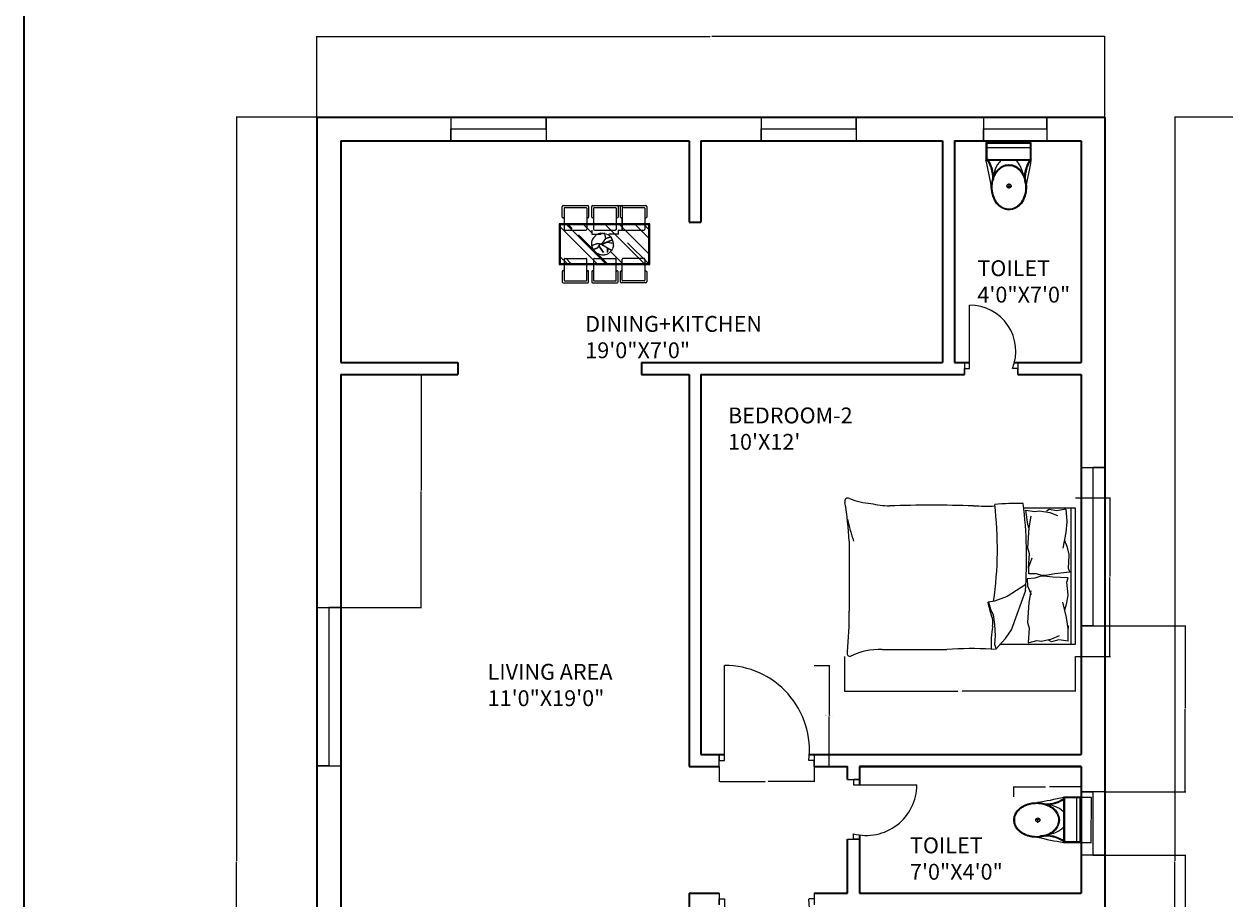
# Model space of a CAD drawing. Units: inches. Extents: x 2416 to 3391, y 1375 to 2496.
# Tile 2 of 13: x 2416 to 2871, y 1738 to 2069. Entities that reach past the tile are written whole.
import ezdxf

# ---------------------------------------------------------------- set-up
doc = ezdxf.new("R2010")
doc.units = ezdxf.units.IN
for name, color, linetype, lineweight in [('A-ANNO-DIMS', 2, 'Continuous', 18), ('A-ANNO-TTLB', 7, 'Continuous', 35), ('A-AREA-IDEN', 7, 'Continuous', 18), ('A-DOOR', 3, 'Continuous', 20), ('A-FLOR-FIXT', 9, 'Continuous', 18), ('A-FURN', 8, 'Continuous', 18), ('A-FURN-PATT', 252, 'Continuous', 13), ('A-GLAZ', 4, 'Continuous', 18), ('A-WALL', 7, 'Continuous', 35)]:
    doc.layers.add(name, color=color, linetype=linetype, lineweight=lineweight)
doc.styles.get("Standard").update_dxf_attribs({"font": 'arial.ttf'})
doc.dimstyles.get("Standard").update_dxf_attribs({"dimtxt": 0.18, "dimasz": 0.18, "dimexe": 0.18, "dimexo": 0.0625, "dimgap": 0.09, "dimtad": 0, "dimtih": 1, "dimtoh": 1, "dimdec": 4, "dimzin": 0, "dimdsep": 46, "dimtxsty": 'Standard', "dimcen": 0.09, "dimadec": 0, "dimazin": 0, "dimtfac": 1, "dimtdec": 4, "dimtofl": 0, "dimtmove": 0, "dimatfit": 3, "dimfxl": 1, "dimtolj": 1, "dimtzin": 0, "dimarcsym": 0})

# ---------------------------------------------------------------- blocks, each defined once
blk = doc.blocks.new('A$C31115884')
for p, q in [((283, 498), (223, 498)), ((258, 466), (258, 523)), ((0, 200), (0, 0)), ((520, 200), (0, 200)), ((10, 190), (10, 10)), ((510, 190), (10, 190)), ((510, 10), (510, 190)), ((520, 0), (520, 200)), ((510, 54), (0, 54)), ((10, 10), (510, 10)), ((0, 0), (520, 0))]:
    blk.add_line(p, q)
blk.add_circle((256, 496), 23.6)
for centre, radius, start, end in [((2778, -205), 2807, 165.4549, 171.7133), ((-295, 403), 365, 324.2091, 9.3499), ((-295, 403), 375, 324.2091, 9.3499), ((139, 406), 293, 315.8436, 2.6563), ((806, 403), 365, 170.6501, 215.7909), ((3237, 905), 2807, 188.2867, 194.5451), ((384, 406), 293, 190.2774, 224.1564), ((806, 403), 375, 179.2036, 215.7909)]:
    blk.add_arc(centre, radius, start, end)
blk.add_ellipse((256, 510), major_axis=(0, -261), ratio=0.772727)
blk.add_open_spline([(256, 259), (263, 259), (270, 260), (288, 262), (299, 265), (320, 273), (330, 278), (350, 291), (360, 299), (378, 316), (386, 326), (402, 347), (409, 358), (421, 383), (427, 395), (436, 422), (440, 436), (445, 465), (447, 480), (448, 509), (448, 524), (445, 553), (443, 568), (436, 596), (432, 610), (422, 636), (416, 649), (402, 672), (395, 683), (379, 703), (370, 712), (351, 728), (341, 735), (321, 746), (310, 751), (289, 757), (278, 759), (256, 761), (245, 761), (223, 757), (212, 754), (191, 746), (181, 741), (161, 728), (151, 720), (133, 703), (125, 693), (110, 672), (103, 660), (90, 636), (85, 623), (76, 596), (72, 582), (67, 553), (66, 538), (64, 509), (65, 494), (68, 465), (70, 450), (77, 422), (81, 408), (91, 382), (97, 370), (111, 346), (118, 335), (135, 316), (144, 307), (162, 291), (172, 284), (193, 273), (203, 269), (225, 262), (236, 260), (250, 259), (253, 259), (256, 259)], degree=3, knots=[0, 0, 0, 0, 0.110105, 0.110105, 0.285049, 0.285049, 0.459994, 0.459994, 0.634938, 0.634938, 0.809882, 0.809882, 0.984827, 0.984827, 1.159771, 1.159771, 1.334715, 1.334715, 1.50966, 1.50966, 1.684604, 1.684604, 1.859549, 1.859549, 2.034493, 2.034493, 2.209437, 2.209437, 2.384382, 2.384382, 2.559326, 2.559326, 2.73427, 2.73427, 2.909215, 2.909215, 3.084159, 3.084159, 3.259103, 3.259103, 3.434048, 3.434048, 3.608992, 3.608992, 3.783936, 3.783936, 3.958881, 3.958881, 4.133825, 4.133825, 4.30877, 4.30877, 4.483714, 4.483714, 4.658658, 4.658658, 4.833603, 4.833603, 5.008547, 5.008547, 5.183491, 5.183491, 5.358436, 5.358436, 5.53338, 5.53338, 5.708324, 5.708324, 5.883269, 5.883269, 6.058213, 6.058213, 6.233158, 6.233158, 6.283185, 6.283185, 6.283185, 6.283185])
blk = doc.blocks.new('WINDOW-60IN')
for p, q in [((0, 60), (9, 60)), ((9, 60), (4.5, 60)), ((4.5, 60), (4.5, 0)), ((4.5, 0), (0, 0)), ((0, 0), (9, 0))]:
    blk.add_line(p, q)
blk = doc.blocks.new('WINDOW-36IN')
for p, q in [((0, 9), (0, 0)), ((36, 4.5), (36, 9)), ((36, 9), (36, 0)), ((0, 0), (0, 4.5)), ((0, 4.5), (36, 4.5))]:
    blk.add_line(p, q)
blk = doc.blocks.new('WINDOW-24IN')
for p, q in [((0, 9), (0, 0)), ((24, 4.5), (24, 9)), ((24, 9), (24, 0)), ((0, 0), (0, 4.5)), ((0, 4.5), (24, 4.5))]:
    blk.add_line(p, q)
blk = doc.blocks.new('DOOR-WC-NORTH')
for p, q in [((0, 0), (0, 24)), ((-2, 2.25), (-2, -2.25)), ((18.23, 2.25), (18.23, -2.25)), ((-2, -2.25), (-2, 0)), ((-2, 0), (0, 0)), ((18.23, 0), (16.23, 0)), ((18.23, -2.25), (18.23, 0))]:
    blk.add_line(p, q)
blk.add_arc((0, 6.51), 17.49, 338.1246, 90)
blk = doc.blocks.new('DOOR-BED-NORTH')
for p, q in [((0, 0), (0, 36)), ((-2, -2.25), (-2, 2.25)), ((-2, 2.25), (-2, 0)), ((33.94, 2.25), (33.94, -2.25)), ((-2, 0), (0, 0)), ((33.94, 0), (31.94, 0)), ((33.94, -2.25), (33.94, 0))]:
    blk.add_line(p, q)
blk.add_arc((0, 3.83), 32.17, 353.1657, 90)
blk = doc.blocks.new('DOOR-BED-SOUTH')
for p, q in [((-2, 2.25), (-2, -2.25)), ((33.94, 2.25), (33.94, -2.25)), ((-2, -2.25), (-2, 0)), ((-2, 0), (0, 0)), ((0, 0), (0, -36)), ((33.94, 0), (31.94, 0))]:
    blk.add_line(p, q)
blk.add_arc((0, -3.83), 32.17, 270, 6.8343)
blk = doc.blocks.new('DOOR-WC-SOUTH')
for p, q in [((-2.25, 2), (2.25, 2)), ((2.25, 2), (0, 2)), ((0, 2), (0, 0)), ((0, 0), (24, 0)), ((-2.25, -20.51), (2.25, -20.51)), ((0, -20.51), (0, -18.51)), ((2.25, -20.51), (0, -20.51))]:
    blk.add_line(p, q)
blk.add_arc((4.87, 0), 19.13, 255.2686, 0)
blk = doc.blocks.new('BED-PILLOWS-PLAN')
for p, q in [((67.77, 56.25), (87.35, 56.25)), ((69.39, 49.97), (68.6, 55.48)), ((68.6, 55.48), (72.04, 54.86)), ((72.04, 54.86), (73.76, 55.17)), ((73.76, 55.17), (77.67, 54.55)), ((77.51, 55.64), (76.42, 55.02)), ((80.33, 55.17), (77.51, 55.64)), ((83.77, 55.8), (80.33, 55.17)), ((83.74, 55.79), (84.1, 51.16)), ((85.69, 56.25), (85.69, 4.59)), ((87.35, 56.25), (87.35, 4.59)), ((70.46, 53.11), (69.74, 48.75)), ((77.67, 54.55), (80.64, 53.45)), ((84.08, 51.05), (83.77, 46.92)), ((84.1, 51.16), (84.08, 51.05)), ((69.74, 48.75), (69.27, 41.17)), ((69.74, 48.75), (69.39, 49.97)), ((83.77, 46.92), (82.67, 40.98)), ((1.68, 43.72), (1.68, 17.11)), ((69.27, 41.17), (69.87, 39.05)), ((83.3, 43.95), (84.08, 41.76)), ((84.08, 41.76), (84.86, 38.64)), ((69.87, 39.05), (69.44, 33.5)), ((69.77, 33.95), (70.95, 37.35)), ((84.86, 38.29), (84.7, 33.48)), ((84.86, 38.64), (84.86, 38.29)), ((69.77, 31.29), (69.77, 33.95)), ((85.33, 31.92), (79.55, 31.29)), ((84.7, 33.48), (85.33, 31.92)), ((68.56, 27.3), (61.54, 22.77)), ((71.98, 29.6), (69.09, 29.42)), ((69.09, 29.42), (69.25, 26.77)), ((72.67, 31.29), (69.77, 31.29)), ((73.97, 30.35), (71.98, 29.6)), ((74.7, 30.67), (72.67, 31.29)), ((75.38, 30.44), (73.97, 30.35)), ((76.11, 30.67), (74.7, 30.67)), ((78.85, 30.03), (75.38, 30.44)), ((79.55, 31.29), (76.11, 30.67)), ((84.66, 29.76), (78.85, 30.03)), ((84.13, 28.16), (84.66, 29.76)), ((84.59, 23.38), (84.13, 28.16)), ((61.54, 22.77), (56.69, 20.92)), ((65.39, 16.07), (68.56, 25.08)), ((69.25, 26.77), (70.64, 23.45)), ((70.46, 24.8), (69.74, 20.45)), ((84.02, 19.86), (84.61, 23.03)), ((84.61, 23.03), (84.59, 23.38)), ((56.69, 20.92), (54.51, 20.59)), ((54.51, 20.59), (55.18, 17.91)), ((69.74, 20.45), (69.27, 12.87)), ((84.03, 14.7), (82.57, 20.55)), ((83.38, 17.63), (84.02, 19.86)), ((55.18, 17.91), (56.19, 15.73)), ((56.19, 15.73), (56.69, 12.05)), ((63.21, 10.04), (65.39, 16.07)), ((84.6, 10.59), (84.03, 14.7)), ((56.69, 12.05), (57.02, 7.87)), ((60.87, 6.86), (63.21, 10.04)), ((69.27, 12.87), (69.87, 10.75)), ((69.87, 10.75), (69.44, 5.2)), ((84.59, 5.83), (84.69, 11.67)), ((84.69, 11.67), (84.6, 10.59)), ((57.02, 7.87), (56.69, 4.52)), ((57.36, 2.86), (60.87, 6.86)), ((87.35, 4.59), (58.58, 4.59)), ((69.44, 5.2), (72.83, 6.04)), ((72.83, 6.04), (74.56, 5.83)), ((74.56, 5.83), (78.42, 6.7)), ((78.34, 5.6), (77.21, 6.16)), ((81.12, 6.24), (78.34, 5.6)), ((78.42, 6.7), (81.32, 7.98)), ((84.59, 5.83), (81.12, 6.24)), ((55.47, 2.77), (57.36, 2.86, 4.18)), ((56.69, 4.52), (57.36, 2.86))]:
    blk.add_line(p, q)
for centre, radius, start, end in [((1.17, 58.83), 1.18, 56.1736, 203.4781), ((11.38, 83.42), 25.47, 247.9751, 266.652), ((-129.76, 36.84), 131.62, 2.9958, 9.4091), ((17.61, 89.09), 32.04, 256.0648, 268.9113), ((32.64, -464.1), 521.39, 88.2277, 91.7185), ((53.65, 240.87), 183.89, 268.4762, 271.0082), ((-81.63, 40.81), 139.47, 351.7845, 6.9006), ((65.63, -32.06), 90.06, 88.7218, 95.604), ((-109.45, 36.92), 178.34, 356.0865, 6.7821), ((112.98, 78.62), 115.08, 193.3832, 197.7053), ((54.44, 20.4), 0.199, 70.2464, 181.1377), ((85.75, 26.33), 32.06, 190.6617, 199.8806), ((-142.13, 15.52), 143.82, 354.4998, 0.6351), ((49.44, 12.72), 6.73, 348.6608, 23.7384), ((94.55, 4.52), 39.11, 169.8763, 182.5657), ((2.09, 1.19), 1.19, 152.6588, 266.02), ((13.12, -22.32), 24.93, 87.4714, 116.4681), ((14.03, 4934.07), 4931.49, 270.00217, 270.28689), ((48.09, -137.03), 139.99, 86.9791, 93.8365)]:
    blk.add_arc(centre, radius, start, end)
blk = doc.blocks.new('CHAIR-DINING')
for p, q in [((0.31, 9.26), (9.67, 9.26)), ((0, 4.94), (0, 8.95)), ((0.31, 4.63), (0.38, 4.63)), ((0.69, 8.26), (0.69, 0.31)), ((1, 8.57), (8.98, 8.57)), ((9.29, 8.26), (9.29, 0.31)), ((9.6, 4.63), (9.67, 4.63)), ((9.98, 8.95), (9.98, 4.94)), ((1, 0), (8.98, 0))]:
    blk.add_line(p, q)
for centre, start, end in [((0.31, 8.95), 90, 180), ((9.67, 8.95), 0, 90), ((0.31, 4.94), 180, 270), ((0.38, 4.94), 270, 0), ((1, 8.26), 90, 180), ((8.98, 8.26), 0, 90), ((9.6, 4.94), 180, 270), ((9.67, 4.94), 270, 0), ((1, 0.31), 180, 270), ((8.98, 0.31), 270, 0)]:
    blk.add_arc(centre, 0.31, start, end)
blk = doc.blocks.new('*D25')
at = {"layer": 'A-ANNO-DIMS', "color": 0, "lineweight": -2, "transparency": 16777216}
for p, q in [((2791.46, 1776.62), (2791.46, 1780.56)), ((2791.64, 1780.38), (2803.43, 1780.38)), ((2816.76, 1780.38), (2804.98, 1780.38)), ((2816.94, 1776.62), (2816.94, 1780.56))]:
    blk.add_line(p, q, dxfattribs=at)
at = {"layer": 'A-ANNO-DIMS', "color": 0, "transparency": 16777216}
for points in [[(2791.64, 1780.41), (2791.64, 1780.35), (2791.46, 1780.38)], [(2816.76, 1780.41), (2816.76, 1780.35), (2816.94, 1780.38)]]:
    blk.add_solid(points, dxfattribs=at)
at = {"layer": 'Defpoints', "color": 0, "transparency": 16777216}
for p in [(2791.46, 1780.38), (2791.46, 1776.56), (2816.94, 1776.56)]:
    blk.add_point(p, dxfattribs=at)
at = {"layer": 'A-ANNO-DIMS', "color": 0, "transparency": 16777216, "insert": (2804.2, 1780.38), "char_height": 0.18, "attachment_point": 5}
blk.add_mtext('\\A1;WC 25 TYP.', dxfattribs=at)
blk = doc.blocks.new('*D26')
at = {"layer": 'A-ANNO-DIMS', "color": 0, "lineweight": -2, "transparency": 16777216}
for p, q in [((2817, 1776.56), (2820.94, 1776.56)), ((2820.76, 1776.38), (2820.76, 1768.14)), ((2820.76, 1759.55), (2820.76, 1767.78)), ((2817, 1759.37), (2820.94, 1759.37))]:
    blk.add_line(p, q, dxfattribs=at)
at = {"layer": 'A-ANNO-DIMS', "color": 0, "transparency": 16777216}
for points in [[(2820.73, 1776.38), (2820.79, 1776.38), (2820.76, 1776.56)], [(2820.73, 1759.55), (2820.79, 1759.55), (2820.76, 1759.37)]]:
    blk.add_solid(points, dxfattribs=at)
at = {"layer": 'Defpoints', "color": 0, "transparency": 16777216}
for p in [(2816.94, 1776.56), (2820.76, 1776.56), (2816.94, 1759.37)]:
    blk.add_point(p, dxfattribs=at)
at = {"layer": 'A-ANNO-DIMS', "color": 0, "transparency": 16777216, "insert": (2820.76, 1767.96), "char_height": 0.18, "attachment_point": 5}
blk.add_mtext('\\A1;17 TYP.', dxfattribs=at)
blk = doc.blocks.new('*D31')
at = {"layer": 'A-ANNO-DIMS', "color": 0, "lineweight": -2, "transparency": 16777216}
for p, q in [((2715.88, 1826.42), (2721.73, 1826.42)), ((2721.55, 1826.24), (2721.55, 1807.48)), ((2721.55, 1788.35), (2721.55, 1807.11)), ((2715.88, 1788.17), (2721.73, 1788.17))]:
    blk.add_line(p, q, dxfattribs=at)
at = {"layer": 'A-ANNO-DIMS', "color": 0, "transparency": 16777216}
for points in [[(2721.52, 1826.24), (2721.58, 1826.24), (2721.55, 1826.42)], [(2721.52, 1788.35), (2721.58, 1788.35), (2721.55, 1788.17)]]:
    blk.add_solid(points, dxfattribs=at)
at = {"layer": 'Defpoints', "color": 0, "transparency": 16777216}
for p in [(2715.81, 1826.42), (2721.55, 1826.42), (2715.81, 1788.17)]:
    blk.add_point(p, dxfattribs=at)
at = {"layer": 'A-ANNO-DIMS', "color": 0, "transparency": 16777216, "insert": (2721.55, 1807.3), "char_height": 0.18, "attachment_point": 5}
blk.add_mtext('\\A1;BEDROOM 2 DOOR 38 TYP.', dxfattribs=at)
blk = doc.blocks.new('*D32')
at = {"layer": 'A-ANNO-DIMS', "color": 0, "lineweight": -2, "transparency": 16777216}
for p, q in [((2679.87, 1788.11), (2679.87, 1782.25)), ((2715.81, 1788.11), (2715.81, 1782.25)), ((2680.05, 1782.43), (2697.31, 1782.43)), ((2715.63, 1782.43), (2698.37, 1782.43))]:
    blk.add_line(p, q, dxfattribs=at)
at = {"layer": 'A-ANNO-DIMS', "color": 0, "transparency": 16777216}
for points in [[(2680.05, 1782.46), (2680.05, 1782.4), (2679.87, 1782.43)], [(2715.63, 1782.46), (2715.63, 1782.4), (2715.81, 1782.43)]]:
    blk.add_solid(points, dxfattribs=at)
at = {"layer": 'Defpoints', "color": 0, "transparency": 16777216}
for p in [(2679.87, 1788.17), (2715.81, 1788.17), (2715.81, 1782.43)]:
    blk.add_point(p, dxfattribs=at)
at = {"layer": 'A-ANNO-DIMS', "color": 0, "transparency": 16777216, "insert": (2697.84, 1782.43), "char_height": 0.18, "attachment_point": 5}
blk.add_mtext('\\A1;36 TYP.', dxfattribs=at)
blk = doc.blocks.new('*D39')
at = {"layer": 'A-ANNO-DIMS', "color": 0, "lineweight": -2, "transparency": 16777216}
for p, q in [((2727.28, 1829.74), (2727.28, 1816.5)), ((2814.75, 1829.74), (2814.75, 1816.5)), ((2727.46, 1816.68), (2770.2, 1816.68)), ((2814.57, 1816.68), (2771.83, 1816.68))]:
    blk.add_line(p, q, dxfattribs=at)
at = {"layer": 'A-ANNO-DIMS', "color": 0, "transparency": 16777216}
for points in [[(2727.46, 1816.71), (2727.46, 1816.65), (2727.28, 1816.68)], [(2814.57, 1816.71), (2814.57, 1816.65), (2814.75, 1816.68)]]:
    blk.add_solid(points, dxfattribs=at)
at = {"layer": 'Defpoints', "color": 0, "transparency": 16777216}
for p in [(2727.28, 1829.8), (2814.75, 1829.8), (2814.75, 1816.68)]:
    blk.add_point(p, dxfattribs=at)
at = {"layer": 'A-ANNO-DIMS', "color": 0, "transparency": 16777216, "insert": (2771.01, 1816.68), "char_height": 0.18, "attachment_point": 5}
blk.add_mtext('\\A1;BED 87 TYP.', dxfattribs=at)
blk = doc.blocks.new('*D40')
at = {"layer": 'A-ANNO-DIMS', "color": 0, "lineweight": -2, "transparency": 16777216}
for p, q in [((2814.81, 1889.9), (2828.05, 1889.9)), ((2827.87, 1889.72), (2827.87, 1860.04)), ((2827.87, 1829.98), (2827.87, 1859.67)), ((2814.81, 1829.8), (2828.05, 1829.8))]:
    blk.add_line(p, q, dxfattribs=at)
at = {"layer": 'A-ANNO-DIMS', "color": 0, "transparency": 16777216}
for points in [[(2827.84, 1889.72), (2827.9, 1889.72), (2827.87, 1889.9)], [(2827.84, 1829.98), (2827.9, 1829.98), (2827.87, 1829.8)]]:
    blk.add_solid(points, dxfattribs=at)
at = {"layer": 'Defpoints', "color": 0, "transparency": 16777216}
for p in [(2814.75, 1889.9), (2827.87, 1889.9), (2814.75, 1829.8)]:
    blk.add_point(p, dxfattribs=at)
at = {"layer": 'A-ANNO-DIMS', "color": 0, "transparency": 16777216, "insert": (2827.87, 1859.85), "char_height": 0.18, "attachment_point": 5}
blk.add_mtext('\\A1;60 TYP.', dxfattribs=at)
blk = doc.blocks.new('*D41')
at = {"layer": 'A-ANNO-DIMS', "color": 0, "lineweight": -2, "transparency": 16777216}
for p, q in [((2631.56, 1991.27), (2631.56, 1989.66)), ((2641.54, 1991.27), (2641.54, 1989.66)), ((2631.74, 1989.84), (2635.12, 1989.84)), ((2641.36, 1989.84), (2637.97, 1989.84))]:
    blk.add_line(p, q, dxfattribs=at)
at = {"layer": 'A-ANNO-DIMS', "color": 0, "transparency": 16777216}
for points in [[(2631.74, 1989.87), (2631.74, 1989.81), (2631.56, 1989.84)], [(2641.36, 1989.87), (2641.36, 1989.81), (2641.54, 1989.84)]]:
    blk.add_solid(points, dxfattribs=at)
at = {"layer": 'Defpoints', "color": 0, "transparency": 16777216}
for p in [(2631.56, 1991.34), (2641.54, 1991.34), (2641.54, 1989.84)]:
    blk.add_point(p, dxfattribs=at)
at = {"layer": 'A-ANNO-DIMS', "color": 0, "transparency": 16777216, "insert": (2636.55, 1989.84), "char_height": 0.18, "attachment_point": 5}
blk.add_mtext('\\A1;DINING CHAIR 10 TYP.', dxfattribs=at)
blk = doc.blocks.new('*D42')
at = {"layer": 'A-ANNO-DIMS', "color": 0, "lineweight": -2, "transparency": 16777216}
for p, q in [((2641.6, 2000.59), (2643.22, 2000.59)), ((2643.04, 2000.41), (2643.04, 1996.15)), ((2643.04, 1991.52), (2643.04, 1995.78)), ((2641.6, 1991.34), (2643.22, 1991.34))]:
    blk.add_line(p, q, dxfattribs=at)
at = {"layer": 'A-ANNO-DIMS', "color": 0, "transparency": 16777216}
for points in [[(2643.01, 2000.41), (2643.07, 2000.41), (2643.04, 2000.59)], [(2643.01, 1991.52), (2643.07, 1991.52), (2643.04, 1991.34)]]:
    blk.add_solid(points, dxfattribs=at)
at = {"layer": 'Defpoints', "color": 0, "transparency": 16777216}
for p in [(2641.54, 2000.59), (2643.04, 2000.59), (2641.54, 1991.34)]:
    blk.add_point(p, dxfattribs=at)
at = {"layer": 'A-ANNO-DIMS', "color": 0, "transparency": 16777216, "insert": (2643.04, 1995.96), "char_height": 0.18, "attachment_point": 5}
blk.add_mtext('\\A1;9 TYP.', dxfattribs=at)
blk = doc.blocks.new('*D47')
at = {"layer": 'A-ANNO-DIMS', "color": 0, "lineweight": -2, "transparency": 16777216}
for p, q in [((2527.44, 2034.23), (2527.44, 2064.8)), ((2527.62, 2064.62), (2676.3, 2064.62)), ((2825.76, 2064.62), (2677.09, 2064.62)), ((2825.94, 2034.23), (2825.94, 2064.8))]:
    blk.add_line(p, q, dxfattribs=at)
at = {"layer": 'A-ANNO-DIMS', "color": 0, "transparency": 16777216}
for points in [[(2527.62, 2064.65), (2527.62, 2064.59), (2527.44, 2064.62)], [(2825.76, 2064.65), (2825.76, 2064.59), (2825.94, 2064.62)]]:
    blk.add_solid(points, dxfattribs=at)
at = {"layer": 'Defpoints', "color": 0, "transparency": 16777216}
for p in [(2825.94, 2064.62), (2527.44, 2034.17), (2825.94, 2034.17)]:
    blk.add_point(p, dxfattribs=at)
at = {"layer": 'A-ANNO-DIMS', "color": 0, "transparency": 16777216, "insert": (2676.69, 2064.62), "char_height": 0.18, "attachment_point": 5}
blk.add_mtext('\\A1;298.5', dxfattribs=at)
blk = doc.blocks.new('*D48')
at = {"layer": 'A-ANNO-DIMS', "color": 0, "lineweight": -2, "transparency": 16777216}
for p, q in [((2527.38, 2034.17), (2496.81, 2034.17)), ((2496.99, 2033.99), (2496.99, 1752.35)), ((2496.99, 1470.35), (2496.99, 1751.99)), ((2527.38, 1470.17), (2496.81, 1470.17))]:
    blk.add_line(p, q, dxfattribs=at)
at = {"layer": 'A-ANNO-DIMS', "color": 0, "transparency": 16777216}
for points in [[(2496.96, 2033.99), (2497.02, 2033.99), (2496.99, 2034.17)], [(2496.96, 1470.35), (2497.02, 1470.35), (2496.99, 1470.17)]]:
    blk.add_solid(points, dxfattribs=at)
at = {"layer": 'Defpoints', "color": 0, "transparency": 16777216}
for p in [(2496.99, 2034.17), (2527.44, 2034.17), (2527.44, 1470.17)]:
    blk.add_point(p, dxfattribs=at)
at = {"layer": 'A-ANNO-DIMS', "color": 0, "transparency": 16777216, "insert": (2496.99, 1752.17), "char_height": 0.18, "attachment_point": 5}
blk.add_mtext('\\A1;564', dxfattribs=at)
blk = doc.blocks.new('*D50')
at = {"layer": 'A-ANNO-DIMS', "color": 0, "lineweight": -2, "transparency": 16777216}
for p, q in [((2536.5, 1936.67), (2567.07, 1936.67)), ((2566.89, 1936.49), (2566.89, 1892.71)), ((2566.89, 1848.56), (2566.89, 1892.35)), ((2536.5, 1848.38), (2567.07, 1848.38))]:
    blk.add_line(p, q, dxfattribs=at)
at = {"layer": 'A-ANNO-DIMS', "color": 0, "transparency": 16777216}
for points in [[(2566.86, 1936.49), (2566.92, 1936.49), (2566.89, 1936.67)], [(2566.86, 1848.56), (2566.92, 1848.56), (2566.89, 1848.38)]]:
    blk.add_solid(points, dxfattribs=at)
at = {"layer": 'Defpoints', "color": 0, "transparency": 16777216}
for p in [(2536.44, 1936.67), (2536.44, 1848.38), (2566.89, 1848.38)]:
    blk.add_point(p, dxfattribs=at)
at = {"layer": 'A-ANNO-DIMS', "color": 0, "transparency": 16777216, "insert": (2566.89, 1892.53), "char_height": 0.18, "attachment_point": 5}
blk.add_mtext('\\A1;88.29', dxfattribs=at)
blk = doc.blocks.new('*D52')
at = {"layer": 'A-ANNO-DIMS', "color": 0, "lineweight": -2, "transparency": 16777216}
for p, q in [((2826, 1754.58), (2856.57, 1754.58)), ((2856.39, 1754.4), (2856.39, 1726.7)), ((2856.39, 1698.63), (2856.39, 1726.33)), ((2826, 1698.45), (2856.57, 1698.45))]:
    blk.add_line(p, q, dxfattribs=at)
at = {"layer": 'A-ANNO-DIMS', "color": 0, "transparency": 16777216}
for points in [[(2856.36, 1754.4), (2856.42, 1754.4), (2856.39, 1754.58)], [(2856.36, 1698.63), (2856.42, 1698.63), (2856.39, 1698.45)]]:
    blk.add_solid(points, dxfattribs=at)
at = {"layer": 'Defpoints', "color": 0, "transparency": 16777216}
for p in [(2825.94, 1754.58), (2825.94, 1698.45), (2856.39, 1698.45)]:
    blk.add_point(p, dxfattribs=at)
at = {"layer": 'A-ANNO-DIMS', "color": 0, "transparency": 16777216, "insert": (2856.39, 1726.51), "char_height": 0.18, "attachment_point": 5}
blk.add_mtext('\\A1;56.14', dxfattribs=at)
blk = doc.blocks.new('*D53')
at = {"layer": 'A-ANNO-DIMS', "color": 0, "lineweight": -2, "transparency": 16777216}
for p, q in [((2826, 1841.41), (2856.57, 1841.41)), ((2856.39, 1841.23), (2856.39, 1810.18)), ((2856.39, 1778.76), (2856.39, 1809.81)), ((2826, 1778.58), (2856.57, 1778.58))]:
    blk.add_line(p, q, dxfattribs=at)
at = {"layer": 'A-ANNO-DIMS', "color": 0, "transparency": 16777216}
for points in [[(2856.36, 1841.23), (2856.42, 1841.23), (2856.39, 1841.41)], [(2856.36, 1778.76), (2856.42, 1778.76), (2856.39, 1778.58)]]:
    blk.add_solid(points, dxfattribs=at)
at = {"layer": 'Defpoints', "color": 0, "transparency": 16777216}
for p in [(2825.94, 1841.41), (2825.94, 1778.58), (2856.39, 1778.58)]:
    blk.add_point(p, dxfattribs=at)
at = {"layer": 'A-ANNO-DIMS', "color": 0, "transparency": 16777216, "insert": (2856.39, 1810), "char_height": 0.18, "attachment_point": 5}
blk.add_mtext('\\A1;62.83', dxfattribs=at)
blk = doc.blocks.new('*D55')
at = {"layer": 'A-ANNO-DIMS', "color": 0, "lineweight": -2, "transparency": 16777216}
for p, q in [((2904.13, 2034.17), (2852.3, 2034.17)), ((2852.48, 2033.99), (2852.48, 1752.35)), ((2852.48, 1470.35), (2852.48, 1751.99)), ((2904.13, 1470.17), (2852.3, 1470.17))]:
    blk.add_line(p, q, dxfattribs=at)
at = {"layer": 'A-ANNO-DIMS', "color": 0, "transparency": 16777216}
for points in [[(2852.45, 2033.99), (2852.51, 2033.99), (2852.48, 2034.17)], [(2852.45, 1470.35), (2852.51, 1470.35), (2852.48, 1470.17)]]:
    blk.add_solid(points, dxfattribs=at)
at = {"layer": 'Defpoints', "color": 0, "transparency": 16777216}
for p in [(2852.48, 2034.17), (2904.19, 2034.17), (2904.19, 1470.17)]:
    blk.add_point(p, dxfattribs=at)
at = {"layer": 'A-ANNO-DIMS', "color": 0, "transparency": 16777216, "insert": (2852.48, 1752.17), "char_height": 0.18, "attachment_point": 5}
blk.add_mtext('\\A1;564', dxfattribs=at)

msp = doc.modelspace()

# ---------------------------------------------------------------- hatches: boundary and pattern name
at = {"layer": 'A-FURN-PATT'}
h = msp.add_hatch(dxfattribs=at)
h.set_pattern_fill('AR-RROOF', color=256, scale=10.323732, angle=-45, style=0)
h.set_pattern_definition([(315, (2958.933, 2853.686), (23.35994, -8.75998), [154.856, -20.6475, 51.6187, -10.3237]), (315, (2972.292, 2847.627), (2.409, 17.00896), [30.9712, -3.4068, 61.9424, -7.7428]), (315, (2968.788, 2856.241), (42.85089, -33.068914), [82.58986, -14.45322, 41.29493, -10.32373])])
h.paths.add_polyline_path([(2619.6069, 1978.6669), (2653.159, 1978.6669), (2653.159, 1993.2922), (2619.6069, 1993.2922)])

# ---------------------------------------------------------------- linework, layer by layer
at = {"layer": 'A-ANNO-TTLB'}
msp.add_lwpolyline([(2416.4678, 2496.0939), (3391.2022, 2496.0939), (3391.2022, 1375.1104), (2416.4678, 1375.1104)], close=True, dxfattribs=at)
at = {"layer": 'A-FURN'}
for p, q in [((2620.7069, 2000.5928), (2630.0671, 2000.5928)), ((2620.3972, 1996.2738), (2620.3972, 2000.283)), ((2620.7069, 1995.9641), (2620.7758, 1995.9641)), ((2621.0855, 1999.5948), (2621.0855, 1991.6451)), ((2621.3952, 1999.9045), (2629.3789, 1999.9045)), ((2629.6886, 1999.5948), (2629.6886, 1991.6451)), ((2629.9983, 1995.9641), (2630.0671, 1995.9641)), ((2630.3768, 2000.283), (2630.3768, 1996.2738)), ((2653.5892, 1993.7224), (2619.1767, 1993.7224)), ((2619.1767, 1993.7224), (2619.1767, 1978.2368)), ((2653.159, 1993.2922), (2619.6069, 1993.2922)), ((2619.6069, 1993.2922), (2619.6069, 1978.6669)), ((2621.3952, 1991.3354), (2629.3789, 1991.3354)), ((2653.159, 1978.6669), (2653.159, 1993.2922)), ((2653.5892, 1978.2368), (2653.5892, 1993.7224)), ((2631.7477, 1986.7519), (2631.4095, 1986.815)), ((2631.8167, 1987.0549), (2631.4844, 1987.1443)), ((2631.9091, 1987.3515), (2631.5849, 1987.4668)), ((2632.0246, 1987.64), (2631.7104, 1987.7803)), ((2632.1623, 1987.9186), (2631.8601, 1988.0831)), ((2632.3215, 1988.1855), (2632.0331, 1988.3732)), ((2632.5011, 1988.439), (2632.2283, 1988.6488)), ((2632.7001, 1988.6777), (2632.4446, 1988.9083)), ((2632.9171, 1988.9001), (2632.6805, 1989.1499)), ((2633.151, 1989.1047), (2632.9347, 1989.3724)), ((2633.4002, 1989.2903), (2633.2056, 1989.5741)), ((2633.6631, 1989.4559), (2633.4914, 1989.7541)), ((2633.9383, 1989.6002), (2633.7905, 1989.911)), ((2634.2239, 1989.7226), (2634.101, 1990.044)), ((2634.5183, 1989.8222), (2634.4209, 1990.1522)), ((2634.8195, 1989.8983), (2634.7484, 1990.235)), ((2635.1258, 1989.9506), (2635.0813, 1990.2918)), ((2636.8163, 1988.0878), (2635.1876, 1985.9353)), ((2639.3975, 1987.5958), (2635.1876, 1985.9353)), ((2635.4027, 1985.9661), (2636.9084, 1988.0878)), ((2635.4353, 1989.9787), (2635.4177, 1990.3224)), ((2635.746, 1989.9824), (2635.7554, 1990.3264)), ((2636.0561, 1989.9618), (2636.0924, 1990.304)), ((2636.3635, 1989.9168), (2636.4266, 1990.2551)), ((2636.5397, 1989.6867), (2636.8163, 1988.0878)), ((2636.8777, 1988.1493), (2636.5397, 1989.6867)), ((2636.6665, 1989.8479), (2636.756, 1990.1802)), ((2638.4141, 1988.6413), (2636.8777, 1988.1493)), ((2636.9084, 1988.0878), (2638.4141, 1988.6413)), ((2636.9632, 1989.7555), (2637.0784, 1990.0797)), ((2637.2517, 1989.64), (2637.392, 1989.9542)), ((2637.3472, 1986.7031), (2639.3975, 1987.5958)), ((2637.3472, 1986.7031), (2639.5511, 1986.3658)), ((2637.5302, 1989.5023), (2637.6948, 1989.8045)), ((2637.7971, 1989.3431), (2637.9848, 1989.6315)), ((2638.0507, 1989.1635), (2638.2605, 1989.4363)), ((2638.2894, 1988.9645), (2638.5199, 1989.22)), ((2638.5117, 1988.7475), (2638.7616, 1988.9841)), ((2638.7163, 1988.5136), (2638.984, 1988.7299)), ((2638.902, 1988.2644), (2639.1858, 1988.459)), ((2639.0675, 1988.0014), (2639.3657, 1988.1732)), ((2639.2119, 1987.7263), (2639.5227, 1987.8741)), ((2639.3342, 1987.4407), (2639.6556, 1987.5636)), ((2639.4338, 1987.1463), (2639.7639, 1987.2437)), ((2639.51, 1986.845), (2639.8467, 1986.9162)), ((2631.6822, 1986.1344), (2631.3382, 1986.1438)), ((2631.6859, 1985.8237), (2631.3422, 1985.806)), ((2631.7028, 1986.4444), (2631.3606, 1986.4808)), ((2631.714, 1985.5142), (2631.3728, 1985.4696)), ((2631.7663, 1985.2079), (2631.4296, 1985.1367)), ((2631.8424, 1984.9066), (2631.5124, 1984.8093)), ((2633.7434, 1986.3043), (2631.5617, 1985.5356)), ((2631.5617, 1985.5356), (2633.7434, 1986.2121)), ((2631.942, 1984.6123), (2631.6206, 1984.4893)), ((2632.0644, 1984.3266), (2631.7536, 1984.1788)), ((2632.2087, 1984.0515), (2631.9105, 1983.8797)), ((2632.3743, 1983.7885), (2632.0904, 1983.5939)), ((2633.7127, 1984.6439), (2632.2377, 1983.9674)), ((2632.2377, 1983.9674), (2633.8049, 1984.5824)), ((2632.5599, 1983.5393), (2632.2922, 1983.3231)), ((2632.7645, 1983.3055), (2632.5147, 1983.0689)), ((2632.9869, 1983.0884), (2632.7563, 1982.8329)), ((2633.2256, 1982.8895), (2633.0158, 1982.6167)), ((2633.4791, 1982.7098), (2633.2914, 1982.4214)), ((2633.746, 1982.5507), (2633.5815, 1982.2484)), ((2634.6345, 1986.0891), (2633.7127, 1984.6439)), ((2635.1876, 1985.9661), (2633.7434, 1986.3043)), ((2633.7434, 1986.2121), (2635.372, 1985.8123)), ((2633.8049, 1984.5824), (2634.6653, 1985.9968)), ((2634.0246, 1982.4129), (2633.8842, 1982.0987)), ((2634.313, 1982.2975), (2634.1978, 1981.9732)), ((2636.0173, 1982.8912), (2634.2043, 1985.3204)), ((2634.2965, 1985.3204), (2636.0173, 1982.8912)), ((2634.6097, 1982.205), (2634.5203, 1981.8727)), ((2634.9127, 1982.1361), (2634.8496, 1981.7978)), ((2637.5537, 1984.5394), (2635.2184, 1985.8123)), ((2635.372, 1985.8431), (2637.1868, 1986.6333)), ((2635.4027, 1985.8431), (2638.998, 1983.7522)), ((2636.4567, 1982.1546), (2636.5279, 1981.8179)), ((2636.758, 1982.2308), (2636.8553, 1981.9007)), ((2637.0523, 1982.3303), (2637.1753, 1982.0089)), ((2639.5511, 1986.3658), (2637.1868, 1986.6333)), ((2637.3379, 1982.4527), (2637.4858, 1982.1419)), ((2637.5537, 1982.8604), (2637.5537, 1984.5394)), ((2637.626, 1984.5), (2637.5537, 1982.8604)), ((2637.6131, 1982.5971), (2637.7848, 1982.2989)), ((2638.998, 1983.7522), (2637.626, 1984.5)), ((2637.8761, 1982.7626), (2638.0707, 1982.4788)), ((2638.1253, 1982.9483), (2638.3415, 1982.6806)), ((2638.3591, 1983.1529), (2638.5957, 1982.903)), ((2638.5762, 1983.3752), (2638.8317, 1983.1447)), ((2638.7751, 1983.6139), (2639.0479, 1983.4041)), ((2638.9548, 1983.8675), (2639.2432, 1983.6797)), ((2639.1139, 1984.1344), (2639.4162, 1983.9698)), ((2639.2517, 1984.4129), (2639.5659, 1984.2726)), ((2639.3671, 1984.7014), (2639.6914, 1984.5862)), ((2639.4596, 1984.998), (2639.7919, 1984.9086)), ((2639.5285, 1985.301), (2639.8668, 1985.238)), ((2639.5623, 1986.5387), (2639.9035, 1986.5833)), ((2639.5734, 1985.6085), (2639.9156, 1985.5722)), ((2639.5904, 1986.2293), (2639.934, 1986.2469)), ((2639.5941, 1985.9186), (2639.9381, 1985.9092)), ((2619.1767, 1978.2368), (2653.5892, 1978.2368)), ((2619.6069, 1978.6669), (2653.159, 1978.6669)), ((2621.0855, 1980.314), (2621.0855, 1972.3643)), ((2621.3952, 1980.6238), (2629.3789, 1980.6238)), ((2629.6886, 1972.3643), (2629.6886, 1980.314)), ((2632.2478, 1980.314), (2632.2478, 1972.3643)), ((2632.5575, 1980.6238), (2640.5412, 1980.6238)), ((2635.2202, 1982.0912), (2635.1838, 1981.749)), ((2635.5302, 1982.0705), (2635.5208, 1981.7265)), ((2635.8409, 1982.0742), (2635.8586, 1981.7306)), ((2636.1504, 1982.1023), (2636.1949, 1981.7611)), ((2640.8509, 1972.3643), (2640.8509, 1980.314)), ((2643.0773, 1972.3643), (2643.0773, 1980.314)), ((2651.3707, 1980.6238), (2643.387, 1980.6238)), ((2651.6804, 1980.314), (2651.6804, 1972.3643)), ((2620.3972, 1975.6853), (2620.3972, 1971.6761)), ((2620.709, 1975.993), (2620.7778, 1975.9925)), ((2630.0001, 1975.9314), (2630.069, 1975.931)), ((2630.3768, 1971.6761), (2630.3768, 1975.6853)), ((2631.5595, 1975.6853), (2631.5595, 1971.6761)), ((2631.871, 1975.919), (2631.9399, 1975.9186)), ((2641.1622, 1975.8574), (2641.231, 1975.857)), ((2641.5391, 1971.6761), (2641.5391, 1975.6853)), ((2642.3891, 1971.6761), (2642.3891, 1975.6853)), ((2642.7692, 1975.8468), (2642.7004, 1975.8472)), ((2652.0603, 1975.7852), (2651.9915, 1975.7857)), ((2652.3687, 1975.6853), (2652.3687, 1971.6761)), ((2620.7069, 1971.3664), (2630.0671, 1971.3664)), ((2621.3952, 1972.0546), (2629.3789, 1972.0546)), ((2631.8692, 1971.3664), (2641.2294, 1971.3664)), ((2632.5575, 1972.0546), (2640.5412, 1972.0546)), ((2652.059, 1971.3664), (2642.6988, 1971.3664)), ((2651.3707, 1972.0546), (2643.387, 1972.0546))]:
    msp.add_line(p, q, dxfattribs=at)
for centre, start, end in [((2620.7069, 2000.283), 90, 180), ((2630.0671, 2000.283), 0, 90), ((2620.7069, 1996.2738), 180, 0.103974), ((2621.3952, 1999.5948), 90, 180), ((2629.3789, 1999.5948), 0, 90), ((2629.9983, 1996.2738), 180, 0.103974), ((2621.3952, 1991.6451), 180, 270), ((2629.3789, 1991.6451), 270, 0), ((2621.3952, 1980.314), 90, 180), ((2629.3789, 1980.314), 0, 90), ((2632.5575, 1980.314), 90, 180), ((2640.5412, 1980.314), 0, 90), ((2643.387, 1980.314), 90, 180), ((2651.3707, 1980.314), 0, 90), ((2620.7069, 1975.6833), 89.620247, 179.620246), ((2620.7758, 1975.6828), 359.620246, 89.620247), ((2629.9981, 1975.6217), 89.620247, 179.620246), ((2630.0669, 1975.6213), 359.620246, 89.620247), ((2631.869, 1975.6093), 89.620247, 179.620246), ((2631.9378, 1975.6089), 359.620246, 89.620247), ((2641.1601, 1975.5477), 89.620247, 179.620246), ((2641.229, 1975.5473), 359.620246, 89.620247), ((2642.6983, 1975.5375), 89.620247, 179.620246), ((2642.7671, 1975.5371), 359.620246, 89.620247), ((2651.9895, 1975.4759), 89.620247, 179.620246), ((2652.0583, 1975.4755), 359.620246, 89.620247), ((2620.7069, 1971.6761), 180, 270), ((2621.3952, 1972.3643), 180, 270), ((2629.3789, 1972.3643), 270, 0), ((2630.0671, 1971.6761), 270, 0), ((2631.8692, 1971.6761), 180, 270), ((2632.5575, 1972.3643), 180, 270), ((2640.5412, 1972.3643), 270, 0), ((2641.2294, 1971.6761), 270, 0), ((2642.6988, 1971.6761), 180, 270), ((2643.387, 1972.3643), 180, 270), ((2651.3707, 1972.3643), 270, 0), ((2652.059, 1971.6761), 270, 0)]:
    msp.add_arc(centre, 0.3097, start, end, dxfattribs=at)
at = {"layer": 'A-WALL'}
for p, q in [((2527.4424, 2034.17), (2527.4424, 1470.17)), ((2527.4424, 2034.17), (2825.9424, 2034.17)), ((2825.9424, 2034.17), (2825.9424, 1470.17)), ((2536.4424, 2025.17), (2668.4424, 2025.17)), ((2536.4424, 2025.17), (2536.4424, 1941.17)), ((2668.4424, 2025.17), (2668.4424, 1994.3212)), ((2672.9424, 2025.17), (2672.9424, 1994.3212)), ((2672.9424, 2025.17), (2764.4424, 2025.17)), ((2764.4424, 2025.17), (2764.4424, 1941.17)), ((2768.9424, 2025.17), (2768.9424, 1941.17)), ((2768.9424, 2025.17), (2816.9424, 2025.17)), ((2816.9424, 2025.17), (2816.9424, 1941.17)), ((2668.4424, 1994.3212), (2672.9424, 1994.3212)), ((2536.4424, 1941.17), (2580.7666, 1941.17)), ((2536.4424, 1936.67), (2580.7666, 1936.67)), ((2536.4424, 1936.67), (2536.4424, 1655.9896)), ((2580.7666, 1941.17), (2580.7666, 1936.67)), ((2650.4424, 1941.17), (2650.4424, 1936.67)), ((2650.4424, 1941.17), (2764.4424, 1941.17)), ((2650.4424, 1936.67), (2668.4424, 1936.67)), ((2668.4424, 1936.67), (2668.4424, 1788.17)), ((2672.9424, 1936.67), (2672.9424, 1792.67)), ((2672.9424, 1936.67), (2772.7162, 1936.67)), ((2768.9424, 1941.17), (2774.7162, 1941.17)), ((2791.6733, 1941.17), (2816.9424, 1941.17)), ((2792.9424, 1936.67), (2816.9424, 1936.67)), ((2816.9424, 1936.67), (2816.9424, 1792.67)), ((2672.9424, 1792.67), (2681.8695, 1792.67)), ((2714.0024, 1792.67), (2816.9424, 1792.67)), ((2668.4424, 1788.17), (2679.8695, 1788.17)), ((2715.8125, 1788.17), (2728.4424, 1788.17)), ((2728.4424, 1783.1345), (2728.4424, 1788.17)), ((2816.9424, 1788.17), (2732.9424, 1788.17)), ((2732.9424, 1788.17), (2732.9424, 1781.1345)), ((2732.9424, 1788.17), (2816.9424, 1788.17)), ((2816.9424, 1788.17), (2816.9424, 1740.17)), ((2728.4424, 1740.17), (2728.4424, 1760.6291)), ((2732.9424, 1762.1797), (2732.9424, 1740.17)), ((2668.4424, 1740.17), (2679.8695, 1740.17)), ((2668.4424, 1740.17), (2668.4424, 1591.4896)), ((2715.8125, 1740.17), (2728.4424, 1740.17)), ((2732.9424, 1740.17), (2816.9424, 1740.17))]:
    msp.add_line(p, q, dxfattribs=at)

# ---------------------------------------------------------------- block references
at = {"layer": 'A-DOOR'}
for name, p in [('DOOR-WC-NORTH', (2774.7162, 1938.92)), ('DOOR-BED-NORTH', (2681.8695, 1790.42)), ('DOOR-WC-SOUTH', (2730.6924, 1781.1345)), ('DOOR-BED-SOUTH', (2681.8695, 1737.92))]:
    msp.add_blockref(name, p, dxfattribs=at)
at = {"layer": 'A-FLOR-FIXT', "xscale": 0.0330640103915726, "yscale": 0.0330640103915726, "zscale": 0.0330640103915726}
for p, rotation in [((2798.0671, 2024.4029), 179.9999999999999), ((2816.9424, 1759.3678), 89.99999999999996)]:
    msp.add_blockref('A$C31115884', p, dxfattribs=dict(at, rotation=rotation))
at = {"layer": 'A-FURN'}
for name, p in [('CHAIR-DINING', (2631.56, 1991.335)), ('CHAIR-DINING', (2642.3896, 1991.335)), ('BED-PILLOWS-PLAN', (2727.396, 1829.804))]:
    msp.add_blockref(name, p, dxfattribs=at)
at = {"layer": 'A-GLAZ'}
for name, p in [('WINDOW-36IN', (2578.232, 2025.17)), ('WINDOW-36IN', (2695.7161, 2025.17)), ('WINDOW-24IN', (2780.017, 2025.17)), ('WINDOW-60IN', (2816.942, 1841.41)), ('WINDOW-60IN', (2527.442, 1788.3842))]:
    msp.add_blockref(name, p, dxfattribs=at)
at = {"layer": 'A-GLAZ', "rotation": 270.0000000000002}
msp.add_blockref('WINDOW-24IN', (2816.9423, 1778.581), dxfattribs=at)

# ---------------------------------------------------------------- texts
at = {"layer": 'A-AREA-IDEN', "char_height": 6, "attachment_point": 1}
for s, width, insert in [('TOILET\\P4\'0"X7\'0"', 55.807099, (2777.6457, 1979.8772)), ('DINING+KITCHEN\\P19\'0"X7\'0"', 110.463704, (2629.0978, 1958.7925)), ("BEDROOM-2\\P10'X12'", 129.31457, (2683.1766, 1924.1153)), ('LIVING AREA\\P11\'0"X19\'0"', 183.87304, (2592.0989, 1826.9911)), ('TOILET\\P7\'0"X4\'0"', 64.829937, (2752.1124, 1761.2389))]:
    msp.add_mtext_dynamic_manual_height_columns(s, width=width, gutter_width=12.5, heights=[0], dxfattribs=dict(at, insert=insert))

# ---------------------------------------------------------------- dimensions: what is measured, and where the dimension line sits
at = {"layer": 'A-ANNO-DIMS'}
dim = msp.add_linear_dim(base=(2825.9424, 2064.62), p1=(2527.4424, 2034.17), p2=(2825.9424, 2034.17), dimstyle='Standard', override={"dimdec": 1, "dimlfac": 1, "dimrnd": 0, "dimzin": 0, "dimdsep": 46, "dimlunit": 2}, dxfattribs=at)
dim.commit()
dim.dimension.update_dxf_attribs({"geometry": '*D47', "text_midpoint": (2676.6924, 2064.62)})
for base, p1, p2, angle, override, picture, middle in [((2496.9924, 2034.17), (2527.4424, 1470.17), (2527.4424, 2034.17), 90, {"dimdec": 0, "dimlfac": 1, "dimrnd": 0, "dimzin": 0, "dimdsep": 46, "dimlunit": 2}, '*D48', (2496.9924, 1752.17)), ((2852.4781, 2034.17), (2904.1924, 1470.17), (2904.1924, 2034.17), 90, {"dimdec": 0, "dimlfac": 1, "dimrnd": 0, "dimzin": 0, "dimdsep": 46, "dimlunit": 2}, '*D55', (2852.4781, 1752.17)), ((2566.8924, 1848.3846), (2536.4424, 1936.67), (2536.4424, 1848.3846), 270, {"dimdec": 2, "dimlfac": 1, "dimrnd": 0, "dimzin": 0, "dimdsep": 46, "dimlunit": 2}, '*D50', (2566.8924, 1892.5273)), ((2856.3924, 1778.5813), (2825.9424, 1841.4103), (2825.9424, 1778.5813), 90, {"dimdec": 2, "dimlfac": 1, "dimrnd": 0, "dimzin": 0, "dimdsep": 46, "dimlunit": 2}, '*D53', (2856.3924, 1809.9958)), ((2856.3924, 1698.4455), (2825.9424, 1754.5813), (2825.9424, 1698.4455), 90, {"dimdec": 2, "dimlfac": 1, "dimrnd": 0, "dimzin": 0, "dimdsep": 46, "dimlunit": 2}, '*D52', (2856.3924, 1726.5134))]:
    dim = msp.add_linear_dim(base=base, p1=p1, p2=p2, angle=angle, dimstyle='Standard', override=override, dxfattribs=at)
    dim.commit()
    dim.dimension.update_dxf_attribs({"geometry": picture, "text_midpoint": middle})
for base, p1, p2, angle, text, picture, middle in [((2643.0361, 2000.5928), (2641.5391, 1991.3354), (2641.5391, 2000.5928), 90, '<> TYP.', '*D42', (2643.0361, 1995.9641)), ((2827.8666, 1889.9041), (2814.7468, 1829.8036), (2814.7468, 1889.9041), 90, '<> TYP.', '*D40', (2827.8666, 1859.8539)), ((2721.55, 1826.42), (2715.8125, 1788.17), (2715.8125, 1826.42), 90, 'BEDROOM 2 DOOR <> TYP.', '*D31', (2721.55, 1807.295)), ((2791.4642, 1780.3828), (2816.9424, 1776.5611), (2791.4642, 1776.5611), 180, 'WC <> TYP.', '*D25', (2804.2033, 1780.3828)), ((2820.7641, 1776.5611), (2816.9424, 1759.3678), (2816.9424, 1776.5611), 90, '<> TYP.', '*D26', (2820.7641, 1767.9644))]:
    dim = msp.add_linear_dim(base=base, p1=p1, p2=p2, angle=angle, text=text, dimstyle='Standard', override={"dimdec": 0, "dimlfac": 1, "dimrnd": 0, "dimzin": 0, "dimdsep": 46, "dimlunit": 2}, dxfattribs=at)
    dim.commit()
    dim.dimension.update_dxf_attribs({"geometry": picture, "text_midpoint": middle})
for base, p1, p2, text, picture, middle in [((2641.5391, 1989.8384), (2631.5595, 1991.3354), (2641.5391, 1991.3354), 'DINING CHAIR <> TYP.', '*D41', (2636.5493, 1989.8384)), ((2814.7468, 1816.6838), (2727.2818, 1829.8036), (2814.7468, 1829.8036), 'BED <> TYP.', '*D39', (2771.0143, 1816.6838)), ((2715.8125, 1782.4325), (2679.8695, 1788.17), (2715.8125, 1788.17), '<> TYP.', '*D32', (2697.841, 1782.4325))]:
    dim = msp.add_linear_dim(base=base, p1=p1, p2=p2, text=text, dimstyle='Standard', override={"dimdec": 0, "dimlfac": 1, "dimrnd": 0, "dimzin": 0, "dimdsep": 46, "dimlunit": 2}, dxfattribs=at)
    dim.commit()
    dim.dimension.update_dxf_attribs({"geometry": picture, "text_midpoint": middle})

doc.saveas('drawing.dxf')
